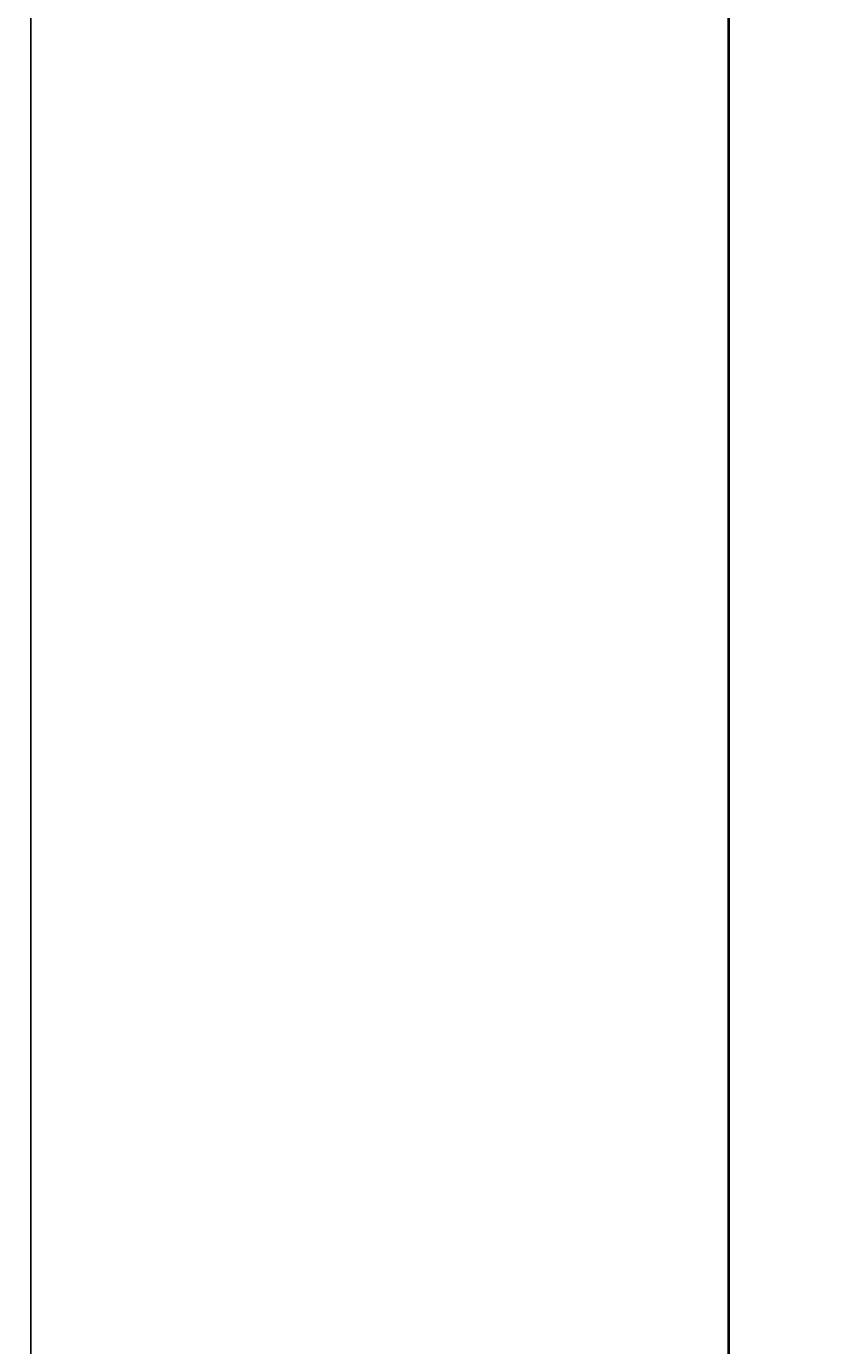
# Model space of a CAD drawing. Units: inches. Extents: x -46 to 1145, y -527 to 760.
# Tile 35 of 57: x -46 to 20, y 541 to 652. Entities that reach past the tile are written whole.
import ezdxf

# ---------------------------------------------------------------- set-up
doc = ezdxf.new("R2010")
doc.units = ezdxf.units.IN
doc.header["$MEASUREMENT"] = 0
doc.layers.add('A-ANNO-DIMS', color=2, linetype='Continuous', lineweight=18)
doc.layers.add('WALLS', color=4, linetype='Continuous', lineweight=40)
doc.styles.get("Standard").update_dxf_attribs({"font": 'arial.ttf'})
doc.dimstyles.get("Standard").update_dxf_attribs({"dimtxt": 0.18, "dimasz": 0.18, "dimexe": 0.18, "dimexo": 0.0625, "dimgap": 0.09, "dimtad": 0, "dimtih": 1, "dimtoh": 1, "dimdec": 0, "dimzin": 0, "dimdsep": 46, "dimlunit": 3, "dimtxsty": 'Standard', "dimcen": 0.09, "dimadec": 0, "dimazin": 0, "dimtfac": 1, "dimtdec": 0, "dimtofl": 0, "dimtmove": 0, "dimatfit": 3, "dimfxl": 1, "dimtolj": 1, "dimtzin": 0, "dimarcsym": 0})

# ---------------------------------------------------------------- blocks, each defined once
blk = doc.blocks.new('*D685')
at = {"layer": 'A-ANNO-DIMS', "color": 0, "lineweight": -2, "transparency": 16777216}
for p, q in [((183.5, 700.89), (-46.22, 700.89)), ((-46.04, 700.71), (-46.04, 116.39)), ((-46.04, -468.3), (-46.04, 116.02)), ((12.5, -468.48), (-46.22, -468.48))]:
    blk.add_line(p, q, dxfattribs=at)
at = {"layer": 'A-ANNO-DIMS', "color": 0, "transparency": 16777216}
for points in [[(-46.07, 700.71), (-46.01, 700.71), (-46.04, 700.89)], [(-46.07, -468.3), (-46.01, -468.3), (-46.04, -468.48)]]:
    blk.add_solid(points, dxfattribs=at)
at = {"layer": 'Defpoints', "color": 0, "transparency": 16777216}
for p in [(-46.04, 700.89), (183.56, 700.89), (12.56, -468.48)]:
    blk.add_point(p, dxfattribs=at)
at = {"layer": 'A-ANNO-DIMS', "color": 0, "transparency": 16777216, "insert": (-46.04, 116.2), "char_height": 0.18, "attachment_point": 5}
blk.add_mtext('\\A1;1169.4', dxfattribs=at)

msp = doc.modelspace()

# ---------------------------------------------------------------- linework, layer by layer
at = {"layer": 'WALLS'}
msp.add_line((12.5637, 659.5176), (12.5637, 221.5176), dxfattribs=at)

# ---------------------------------------------------------------- dimensions: what is measured, and where the dimension line sits
at = {"layer": 'A-ANNO-DIMS'}
dim = msp.add_linear_dim(base=(-46.0363, 700.8886), p1=(12.5637, -468.4824), p2=(183.5637, 700.8886), angle=90, dimstyle='Standard', override={"dimdec": 1, "dimlfac": 1, "dimrnd": 0, "dimzin": 0, "dimdsep": 46, "dimlunit": 2}, dxfattribs=at)
dim.commit()
dim.dimension.update_dxf_attribs({"geometry": '*D685', "text_midpoint": (-46.0363, 116.2031)})

doc.saveas('drawing.dxf')
